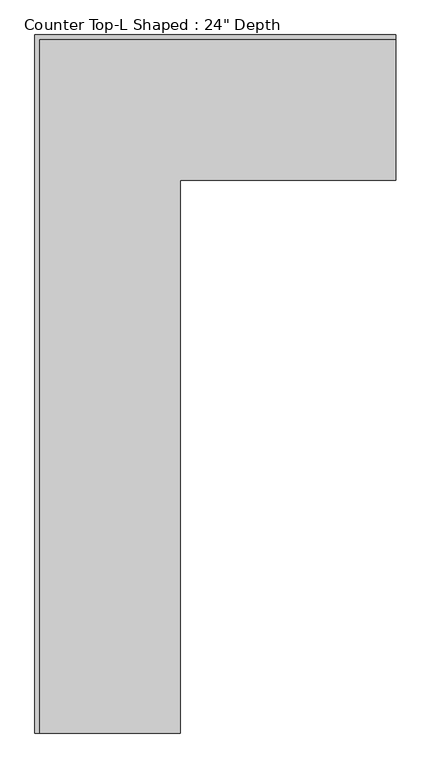
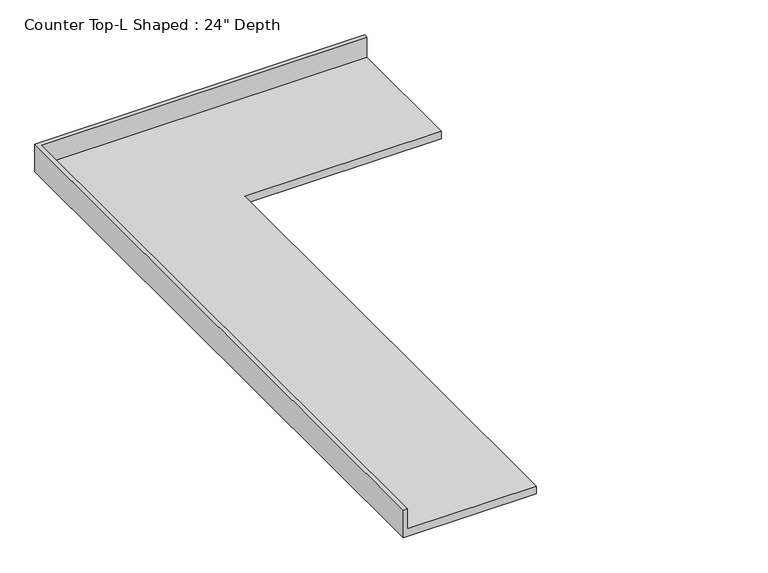
"""IFC4 building model written with IfcOpenShell, lengths in millimetres: furniture geometry."""

from ifc_helpers import new_model, si_unit, origin, place, context, project, spatial, faceted_brep, source, transform, mapped, element, save


def furniture_f6f93809(model_context):
    return source(origin(), model_context, "Body", "Brep", [
        faceted_brep([(-565.4622951, -3048.0, 914.4), (-565.4622951, -635.0, 914.4), (374.3377049, -635.0, 914.4), (374.3377049, -19.05, 914.4), (-1181.4122951, -19.05, 914.4), (-1181.4122951, -3048.0, 914.4), (374.3377049, 0.0, 876.3), (374.3377049, -635.0, 876.3), (-565.4622951, -635.0, 876.3), (-565.4622951, -3048.0, 876.3), (-1200.4622951, -3048.0, 876.3), (-1200.4622951, 0.0, 876.3), (-1200.4622951, 0.0, 1016.0), (374.3377049, 0.0, 1016.0), (-1200.4622951, -3048.0, 1016.0), (-1181.4122951, -3048.0, 1016.0), (374.3377049, -19.05, 1016.0), (-1181.4122951, -19.05, 1016.0)], [[[0, 1, 2, 3, 4, 5]], [[6, 7, 8, 9, 10, 11]], [[6, 11, 12, 13]], [[11, 10, 14, 12]], [[14, 10, 9, 0, 5, 15]], [[1, 0, 9, 8]], [[2, 1, 8, 7]], [[7, 6, 13, 16, 3, 2]], [[12, 14, 15, 17, 16, 13]], [[3, 16, 17, 4]], [[17, 15, 5, 4]]]),
    ])


if __name__ == "__main__":
    model = new_model("IFC4")
    model_context = context("Model", 3, world=origin())
    ifc_project = project(units=[si_unit("LENGTHUNIT", "METRE", prefix="MILLI")], contexts=[model_context])
    site = spatial("IfcSite", under=ifc_project)
    building = spatial("IfcBuilding", under=site)
    placement = place(None, origin())
    furniture_shape = furniture_f6f93809(model_context)
    element("IfcFurniture", 1, ObjectType="Counter Top-L Shaped : 24\" Depth", at=placement, inside=building, context=model_context, shape_type="MappedRepresentation", body=[
        mapped(furniture_shape, transform((0.0, 0.0, 0.0), x_axis=(1.0, 0.0, 0.0), y_axis=(0.0, 1.0, 0.0), z_axis=(0.0, 0.0, 1.0))),
    ])
    save(model, "model.ifc")

# Revit data of these elements
# Type "Counter Top-L Shaped : 24\" Depth"
#   Assembly Code = "C1030400"
#   Counter Thickness = 0' - 1 1/2"
#   Depth = 2' - 1"
#   Height = 3' - 0"
#   Length - Leg 1 [instance default] = 8' - 0"
#   Length - Leg 2 [instance default] = 6' - 0"
#   Counter Top Material = none
#   Default Elevation = 0
# Element 1 (IfcFurniture, "Counter Top-L Shaped : 24\" Depth")
#   Length - Leg 1 = 5' - 2"
#   Length - Leg 2 = 10' - 0"
#   Materials on its faces: "Counter Top"
# Materials
#   "Counter Top": class "Wood", colour RGB 226 177 128, transparency 0
